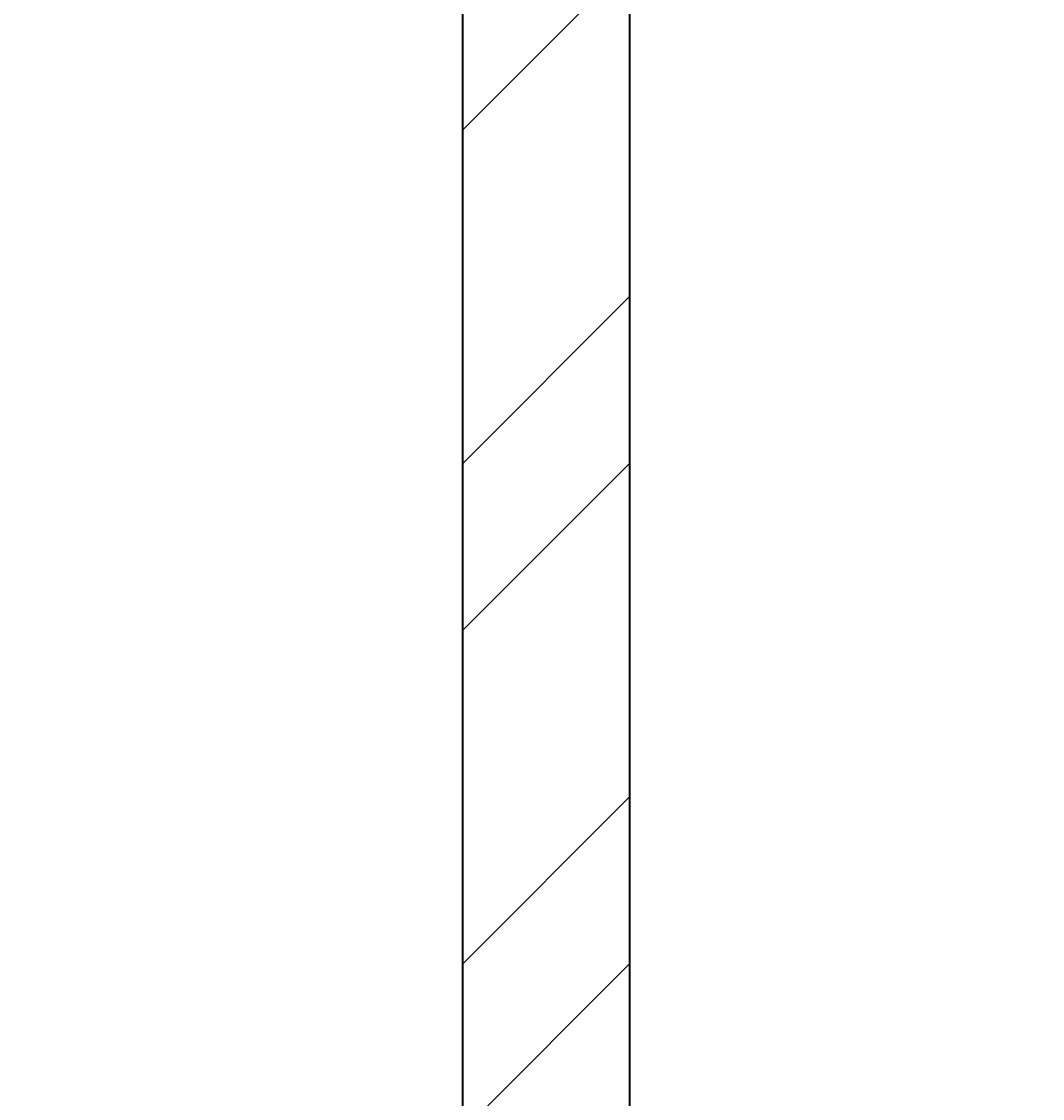
# Model space of a CAD drawing. Units: inches. Extents: x 1962 to 2771, y 1245 to 2660.
# Tile 63 of 114: x 2496 to 2523, y 2033 to 2062. Entities that reach past the tile are written whole.
import ezdxf

# ---------------------------------------------------------------- set-up
doc = ezdxf.new("R2010")
doc.units = ezdxf.units.IN
for name, color, linetype, lineweight in [('A-ANNO-DIMS', 2, 'Continuous', 18), ('A-WALL', 7, 'Continuous', 35), ('A-WALL-PATT', 252, 'Continuous', 13)]:
    doc.layers.add(name, color=color, linetype=linetype, lineweight=lineweight)
doc.styles.get("Standard").update_dxf_attribs({"font": 'arial.ttf'})
doc.dimstyles.get("Standard").update_dxf_attribs({"dimtxt": 0.18, "dimasz": 0.18, "dimexe": 0.18, "dimexo": 0.0625, "dimgap": 0.09, "dimtad": 0, "dimtih": 1, "dimtoh": 1, "dimdec": 4, "dimzin": 0, "dimdsep": 46, "dimtxsty": 'Standard', "dimcen": 0.09, "dimadec": 0, "dimazin": 0, "dimtfac": 1, "dimtdec": 4, "dimtofl": 0, "dimtmove": 0, "dimatfit": 3, "dimfxl": 1, "dimtolj": 1, "dimtzin": 0, "dimarcsym": 0})

# ---------------------------------------------------------------- blocks, each defined once
blk = doc.blocks.new('*D40')
at = {"layer": 'A-ANNO-DIMS', "color": 0, "lineweight": -2, "transparency": 16777216}
for p, q in [((2072.02, 2033.906), (2072.02, 2583.474)), ((2660.807, 2524.406), (2660.807, 2583.474)), ((2072.2, 2583.294), (2366.02, 2583.294)), ((2660.627, 2583.294), (2366.808, 2583.294))]:
    blk.add_line(p, q, dxfattribs=at)
at = {"layer": 'A-ANNO-DIMS', "color": 0, "transparency": 16777216}
for points in [[(2072.2, 2583.324), (2072.2, 2583.264), (2072.02, 2583.294)], [(2660.627, 2583.324), (2660.627, 2583.264), (2660.807, 2583.294)]]:
    blk.add_solid(points, dxfattribs=at)
at = {"layer": 'Defpoints', "color": 0, "transparency": 16777216}
for p in [(2660.807, 2583.294), (2660.807, 2524.344), (2072.02, 2033.844)]:
    blk.add_point(p, dxfattribs=at)
at = {"layer": 'A-ANNO-DIMS', "color": 0, "transparency": 16777216, "insert": (2366.414, 2583.294), "char_height": 0.18, "attachment_point": 5}
blk.add_mtext('\\A1;588.8', dxfattribs=at)

msp = doc.modelspace()

# ---------------------------------------------------------------- hatches: boundary and pattern name
at = {"layer": 'A-WALL-PATT'}
h = msp.add_hatch(dxfattribs=at)
h.set_pattern_fill('ANSI32', color=256)
h.paths.add_polyline_path([(2090.8074, 2467.3437), (2141.6481, 2467.3437), (2141.6481, 2469.5937), (2141.6481, 2471.8437), (2086.3074, 2471.8437), (2086.3074, 2422.5333), (2090.8074, 2422.5333)])
h.paths.add_polyline_path([(2282.7664, 2471.8437), (2204.8982, 2471.8437), (2204.8982, 2467.3437), (2234.8074, 2467.3437), (2234.8074, 2311.3437), (2228.7492, 2311.3437), (2228.7492, 2306.8437), (2234.8074, 2306.8437), (2331.9227, 2306.8437), (2331.9227, 2309.0937), (2331.9227, 2311.3437), (2239.3074, 2311.3437), (2239.3074, 2467.3437), (2282.7664, 2467.3437), (2282.7664, 2469.5937)])
h.paths.add_polyline_path([(2471.4531, 2519.8437), (2552.011, 2519.8437), (2564.3996, 2519.8437), (2564.3996, 2511.1389), (2568.8996, 2511.1389), (2568.8996, 2524.3437), (2466.9531, 2524.3437), (2466.9531, 2471.8437), (2450.0749, 2471.8437), (2446.4672, 2471.8437), (2446.4672, 2467.3437), (2450.0749, 2467.3437), (2475.9988, 2467.3437), (2475.9988, 2469.5937), (2475.9988, 2471.8437), (2471.4531, 2471.8437)])
h.paths.add_polyline_path([(2575.2231, 2469.5937), (2575.2231, 2471.8437), (2568.8996, 2471.8437), (2568.8996, 2487.1389), (2564.3996, 2487.1389), (2564.3996, 2471.8437), (2556.511, 2471.8437), (2499.2904, 2471.8437), (2499.2904, 2467.3437), (2507.8074, 2467.3437), (2507.8074, 2311.3437), (2414.863, 2311.3437), (2414.863, 2306.8437), (2512.3074, 2306.8437), (2517.0114, 2306.8437), (2517.0114, 2309.0937), (2517.0114, 2311.3437), (2512.3074, 2311.3437), (2512.3074, 2467.3437), (2575.2231, 2467.3437)])
h.paths.add_polyline_path([(2660.8074, 2471.8437), (2600.9602, 2471.8437), (2600.9602, 2467.3437), (2656.3074, 2467.3437), (2656.3074, 2432.5704), (2660.8074, 2432.5704)])
h.paths.add_polyline_path([(2660.8074, 2372.5704), (2656.3074, 2372.5704), (2656.3074, 2311.3437), (2600.276, 2311.3437), (2600.276, 2309.0937), (2600.276, 2306.8437), (2656.3074, 2306.8437), (2656.3074, 2296.2593), (2660.8074, 2296.2593)])
h.paths.add_polyline_path([(2572.3074, 2306.8437), (2577.1385, 2306.8437), (2577.1385, 2311.3437), (2551.082, 2311.3437), (2551.082, 2306.8437), (2567.8074, 2306.8437), (2567.8074, 2258.8437), (2540.0574, 2258.8437), (2540.0574, 2256.5937), (2540.0574, 2254.3437), (2567.8074, 2254.3437), (2656.3074, 2254.3437), (2656.3074, 2236.9085), (2660.8074, 2236.9085), (2660.8074, 2272.2593), (2656.3074, 2272.2593), (2656.3074, 2258.8437), (2572.3074, 2258.8437)])
h.paths.add_polyline_path([(2512.3074, 2254.3437), (2518.8716, 2254.3437), (2518.8716, 2256.5937), (2518.8716, 2258.8437), (2507.8074, 2258.8437), (2507.8074, 2177.8437), (2567.8074, 2177.8437), (2567.8074, 2172.9628), (2572.3074, 2172.9628), (2572.3074, 2177.8437), (2656.3074, 2177.8437), (2656.3074, 2166.4846), (2660.8074, 2166.4846), (2660.8074, 2200.9085), (2656.3074, 2200.9085), (2656.3074, 2182.3437), (2512.3074, 2182.3437)])
h.paths.add_polyline_path([(2656.3074, 2129.8437), (2572.3074, 2129.8437), (2572.3074, 2150.3044), (2570.0574, 2150.3044), (2567.8074, 2150.3044), (2567.8074, 2129.8437), (2507.8074, 2129.8437), (2507.8074, 2116.3027), (2510.0574, 2116.3027), (2512.3074, 2116.3027), (2512.3074, 2125.3437), (2567.8074, 2125.3437), (2572.3074, 2125.3437), (2656.3074, 2125.3437)])
h.paths.add_polyline_path([(2090.8074, 2362.5333), (2086.3074, 2362.5333), (2086.3074, 2298.6242), (2090.8074, 2298.6242), (2090.8074, 2306.8437), (2174.8074, 2306.8437), (2174.8074, 2286.4178), (2179.3074, 2286.4178), (2179.3074, 2306.8437), (2192.8641, 2306.8437), (2192.8641, 2309.0937), (2192.8641, 2311.3437), (2090.8074, 2311.3437)])
h.paths.add_polyline_path([(2209.156, 2258.8437), (2179.3074, 2258.8437), (2179.3074, 2263.2236), (2177.0574, 2263.2236), (2174.8074, 2263.2236), (2174.8074, 2258.8437), (2090.8074, 2258.8437), (2090.8074, 2274.6242), (2086.3074, 2274.6242), (2086.3074, 2238.2967), (2088.5574, 2238.2967), (2090.8074, 2238.2967), (2090.8074, 2254.3437), (2209.156, 2254.3437)])
h.paths.add_polyline_path([(2090.8074, 2177.8437), (2234.8074, 2177.8437), (2234.8074, 2173.1428), (2239.3074, 2173.1428), (2239.3074, 2258.8437), (2230.8442, 2258.8437), (2230.8442, 2256.5937), (2230.8442, 2254.3437), (2234.8074, 2254.3437), (2234.8074, 2182.3437), (2090.8074, 2182.3437), (2090.8074, 2202.2967), (2086.3074, 2202.2967), (2086.3074, 2140.0389), (2090.8074, 2140.0389)])
h.paths.add_polyline_path([(2090.8074, 2080.0389), (2086.3074, 2080.0389), (2086.3074, 2033.8437), (2090.8074, 2033.8437)], flags=17)
h.paths.add_polyline_path([(2244.9405, 2033.8437), (2239.3074, 2033.8437), (2239.3074, 2142.0665), (2237.2592, 2142.0665), (2234.8074, 2142.0665), (2234.8074, 2033.8437), (2090.8074, 2033.8437), (2076.5204, 2033.8437), (2072.0204, 2033.8437), (2072.0204, 2000.4493), (2076.5204, 2000.4493), (2076.5204, 2029.3437), (2090.8074, 2029.3437), (2244.9405, 2029.3437), (2244.9405, 2031.5937)])
h.paths.add_polyline_path([(2234.8074, 1933.3437), (2076.5204, 1933.3437), (2076.5204, 1952.4493), (2074.2704, 1952.4493), (2072.0204, 1952.4493), (2072.0204, 1933.3437), (2072.0204, 1928.8437), (2234.8074, 1928.8437)])
h.paths.add_polyline_path([(2090.8074, 1928.8437), (2086.3074, 1928.8437), (2086.3074, 1906.5013), (2090.8074, 1906.5013)])
h.paths.add_polyline_path([(2090.8074, 1846.5013), (2086.3074, 1846.5013), (2086.3074, 1769.9917), (2088.5574, 1769.9917), (2090.8074, 1769.9917), (2090.8074, 1780.3437), (2234.8074, 1780.3437), (2234.8074, 1708.3437), (2230.3764, 1708.3437), (2230.3764, 1703.8437), (2239.3074, 1703.8437), (2239.3074, 1792.6669), (2237.0574, 1792.6669), (2234.8074, 1792.6669), (2234.8074, 1784.8437), (2090.8074, 1784.8437)])
h.paths.add_polyline_path([(2239.3074, 1928.8437), (2244.9405, 1928.8437), (2244.9405, 1931.0937), (2244.9405, 1933.3437), (2234.8074, 1933.3437), (2234.8074, 1928.8437), (2234.8074, 1825.5949), (2239.3074, 1825.5949)])
h.paths.add_polyline_path([(2148.0425, 1649.0937), (2148.0425, 1651.3437), (2090.8074, 1651.3437), (2090.8074, 1646.8437), (2148.0425, 1646.8437)], flags=0)
h.paths.add_polyline_path([(2207.5601, 1708.3437), (2090.8074, 1708.3437), (2090.8074, 1703.8437), (2174.8074, 1703.8437), (2174.8074, 1651.3437), (2170.4457, 1651.3437), (2170.4457, 1646.8437), (2195.9924, 1646.8437), (2195.9924, 1649.0937), (2195.9924, 1651.3437), (2179.3074, 1651.3437), (2179.3074, 1703.8437), (2207.5601, 1703.8437), (2207.5601, 1706.0937)])
h.paths.add_polyline_path([(2090.8074, 1733.9917), (2086.3074, 1733.9917), (2086.3074, 1696.1032), (2088.5574, 1696.1032), (2090.8074, 1696.1032)])
h.paths.add_polyline_path([(2090.8074, 1672.1032), (2086.3074, 1672.1032), (2086.3074, 1600.3335), (2090.8074, 1600.3335)])
h.paths.add_polyline_path([(2090.8074, 1540.3335), (2086.3074, 1540.3335), (2086.3074, 1486.3437), (2139.6766, 1486.3437), (2139.6766, 1490.8437), (2090.8074, 1490.8437)])
h.paths.add_polyline_path([(2302.3876, 1490.8437), (2239.3074, 1490.8437), (2239.3074, 1646.8437), (2335.9994, 1646.8437), (2335.9994, 1651.3437), (2229.884, 1651.3437), (2229.884, 1646.8437), (2234.8074, 1646.8437), (2234.8074, 1490.8437), (2202.7103, 1490.8437), (2202.7103, 1488.5937), (2202.7103, 1486.3437), (2275.0699, 1486.3437), (2275.0699, 1475.772), (2279.5699, 1475.772), (2279.5699, 1486.3437), (2302.3876, 1486.3437)])
h.paths.add_polyline_path([(2279.5699, 1451.772), (2275.0699, 1451.772), (2275.0699, 1438.3437), (2174.8074, 1438.3437), (2174.8074, 1486.3437), (2179.7922, 1486.3437), (2179.7922, 1490.8437), (2163.3585, 1490.8437), (2163.3585, 1488.5937), (2163.3585, 1486.3437), (2170.3074, 1486.3437), (2170.3074, 1433.8437), (2279.5699, 1433.8437)])
h.paths.add_polyline_path([(2427.2363, 1490.8437), (2375.8074, 1490.8437), (2375.8074, 1646.8437), (2381.6401, 1646.8437), (2381.6401, 1651.3437), (2365.887, 1651.3437), (2365.887, 1649.0937), (2365.887, 1646.8437), (2371.3074, 1646.8437), (2371.3074, 1490.8437), (2327.5627, 1490.8437), (2327.5627, 1488.5937), (2327.5627, 1486.3437), (2371.3074, 1486.3437), (2371.3074, 1433.8437), (2375.8074, 1433.8437), (2375.8074, 1486.3437), (2427.2363, 1486.3437)])
h.paths.add_polyline_path([(2512.3074, 1646.8437), (2519.4351, 1646.8437), (2519.4351, 1649.0937), (2519.4351, 1651.3437), (2507.8074, 1651.3437), (2416.0063, 1651.3437), (2416.0063, 1649.0937), (2416.0063, 1646.8437), (2507.8074, 1646.8437), (2507.8074, 1490.8437), (2497.0532, 1490.8437), (2497.0532, 1488.5937), (2497.0532, 1486.3437), (2574.9344, 1486.3437), (2574.9344, 1476.0181), (2579.4344, 1476.0181), (2579.4344, 1486.3437), (2584.4872, 1486.3437), (2584.3074, 1490.8437), (2512.3074, 1490.8437)])
h.paths.add_polyline_path([(2470.5091, 1486.3437), (2473.9767, 1486.3437), (2473.9767, 1490.8437), (2449.6605, 1490.8437), (2449.6605, 1488.5937), (2449.6605, 1486.3437), (2466.0091, 1486.3437), (2466.0091, 1433.8437), (2470.5091, 1433.8437), (2579.4344, 1433.8437), (2579.4344, 1452.0181), (2574.9344, 1452.0181), (2574.9344, 1438.3437), (2554.5091, 1438.3437), (2470.5091, 1438.3437)])
h.paths.add_polyline_path([(2656.3074, 1490.8437), (2611.86, 1490.8437), (2611.86, 1486.3437), (2656.3074, 1486.3437)])
h.paths.add_polyline_path([(2660.8074, 1532.7007), (2658.5574, 1532.7007), (2656.3074, 1532.7007), (2656.3074, 1486.3437), (2660.8074, 1486.3437)])
h.paths.add_polyline_path([(2660.8074, 1664.9663), (2656.3074, 1664.9663), (2656.3074, 1651.3437), (2602.2313, 1651.3437), (2602.2313, 1646.8437), (2656.3074, 1646.8437), (2656.3074, 1592.7007), (2660.8074, 1592.7007)])
h.paths.add_polyline_path([(2660.8074, 1724.5221), (2656.3074, 1724.5221), (2656.3074, 1703.8437), (2542.4725, 1703.8437), (2542.4725, 1699.3437), (2567.8074, 1699.3437), (2567.8074, 1651.3437), (2552.7766, 1651.3437), (2552.7766, 1649.0937), (2552.7766, 1646.8437), (2577.2878, 1646.8437), (2577.2878, 1649.0937), (2577.2878, 1651.3437), (2572.3074, 1651.3437), (2572.3074, 1699.3437), (2656.3074, 1699.3437), (2656.3074, 1688.9663), (2660.8074, 1688.9663)])
h.paths.add_polyline_path([(2660.8074, 1880.6524), (2656.3074, 1880.6524), (2656.3074, 1832.8437), (2512.3074, 1832.8437), (2512.3074, 1837.8959), (2507.8074, 1837.8959), (2507.8074, 1828.3437), (2567.8074, 1828.3437), (2567.8074, 1804.3437), (2572.3074, 1804.3437), (2572.3074, 1828.3437), (2656.3074, 1828.3437), (2656.3074, 1818.6778), (2660.8074, 1818.6778)])
h.paths.add_polyline_path([(2660.8074, 1794.6778), (2656.3074, 1794.6778), (2656.3074, 1780.3437), (2572.3074, 1780.3437), (2572.3074, 1783.0303), (2570.0574, 1783.0303), (2567.8074, 1783.0303), (2567.8074, 1780.3437), (2507.8074, 1780.3437), (2507.8074, 1699.3437), (2517.8858, 1699.3437), (2517.8858, 1701.5937), (2517.8858, 1703.8437), (2512.3074, 1703.8437), (2512.3074, 1775.8437), (2656.3074, 1775.8437), (2656.3074, 1760.5221), (2660.8074, 1760.5221)])
h.paths.add_polyline_path([(2660.8074, 1981.3437), (2660.8074, 2020.2808), (2658.5574, 2020.2808), (2656.3074, 2020.2808), (2656.3074, 1981.3437), (2512.3074, 1981.3437), (2512.3074, 2086.6996), (2507.8074, 2086.6996), (2507.8074, 1981.3437), (2375.8074, 1981.3437), (2375.8074, 1986.8505), (2373.5574, 1986.8505), (2371.3074, 1986.8505), (2371.3074, 1973.2607), (2375.8074, 1973.2607), (2375.8074, 1976.8437), (2507.8074, 1976.8437), (2507.8074, 1865.4281), (2510.0574, 1865.4281), (2512.3074, 1865.4281), (2512.3074, 1976.8437), (2660.8074, 1976.8437)])
h.paths.add_polyline_path([(2375.8074, 1940.297), (2373.5574, 1940.297), (2371.3074, 1940.297), (2371.3074, 1933.3437), (2278.4434, 1933.3437), (2278.4434, 1928.8437), (2371.3074, 1928.8437), (2371.3074, 1651.3437), (2375.8074, 1651.3437)])
h.paths.add_polyline_path([(2660.8074, 1976.8437), (2656.3074, 1976.8437), (2656.3074, 1940.6524), (2660.8074, 1940.6524)], flags=17)
h.paths.add_polyline_path([(2660.8074, 2142.4846), (2656.3074, 2142.4846), (2656.3074, 2080.2808), (2660.8074, 2080.2808)])
h.paths.add_polyline_path([(2381.4189, 2311.3437), (2375.8074, 2311.3437), (2375.8074, 2467.3437), (2424.7242, 2467.3437), (2424.7242, 2469.5937), (2424.7242, 2471.8437), (2375.8074, 2471.8437), (2375.8074, 2524.3437), (2371.3074, 2524.3437), (2371.3074, 2471.8437), (2307.2097, 2471.8437), (2307.2097, 2467.3437), (2371.3074, 2467.3437), (2371.3074, 2311.3437), (2366.8901, 2311.3437), (2366.8901, 2306.8437), (2371.3074, 2306.8437), (2371.3074, 2033.8437), (2279.6589, 2033.8437), (2279.6589, 2029.3437), (2371.3074, 2029.3437), (2371.3074, 2014.2598), (2375.8074, 2014.2598), (2375.8074, 2306.8437), (2381.4189, 2306.8437)])
h.paths.add_polyline_path([(2263.3074, 2524.3437), (2170.3074, 2524.3437), (2170.3074, 2519.8437), (2170.3074, 2471.8437), (2165.0312, 2471.8437), (2165.0312, 2467.3437), (2179.6721, 2467.3437), (2179.6721, 2469.5161), (2179.6721, 2471.8437), (2174.8074, 2471.8437), (2174.8074, 2519.8437), (2258.8074, 2519.8437), (2258.8074, 2511.6436), (2263.3074, 2511.6436)])
h.paths.add_polyline_path([(2245.0232, 1361.4123), (2492.9468, 1361.4123), (2492.9468, 1398.505), (2245.0232, 1398.505)], flags=9)
h.paths.add_polyline_path([(2388.1434, 2086.6936), (2425.0704, 2086.6936), (2425.0704, 2105.3509), (2388.1434, 2105.3509)], flags=9)
h.paths.add_polyline_path([(2404.922, 2242.6744), (2445.7337, 2242.6744), (2445.7337, 2261.3318), (2404.922, 2261.3318)], flags=9)
h.paths.add_polyline_path([(2269.4107, 2156.7935), (2306.3378, 2156.7935), (2306.3378, 2175.4508), (2269.4107, 2175.4508)], flags=9)
h.paths.add_polyline_path([(2269.3277, 2233.4343), (2306.2547, 2233.4343), (2306.2547, 2252.0917), (2269.3277, 2252.0917)], flags=9)
h.paths.add_polyline_path([(2431.6052, 2320.6922), (2470.4456, 2320.6922), (2470.4456, 2339.3495), (2431.6052, 2339.3495)], flags=25)
h.paths.add_polyline_path([(2249.6902, 2315.7608), (2288.5306, 2315.7608), (2288.5306, 2334.4182), (2249.6902, 2334.4182)], flags=25)
h.paths.add_polyline_path([(2096.9301, 2314.3181), (2135.7704, 2314.3181), (2135.7704, 2332.9755), (2096.9301, 2332.9755)], flags=25)
h.paths.add_polyline_path([(2134.3475, 2285.7089), (2161.4655, 2285.7089), (2161.4655, 2304.3662), (2134.3475, 2304.3662)], flags=9)
h.paths.add_polyline_path([(2126.5155, 2209.4076), (2159.9227, 2209.4076), (2159.9227, 2228.065), (2126.5155, 2228.065)], flags=25)
h.paths.add_polyline_path([(2110.5753, 2141.5299), (2149.4157, 2141.5299), (2149.4157, 2160.1872), (2110.5753, 2160.1872)], flags=25)
h.paths.add_polyline_path([(2249.8618, 1968.3317), (2286.3966, 1968.3317), (2286.3966, 1986.989), (2249.8618, 1986.989)], flags=9)
h.paths.add_polyline_path([(2395.9507, 1777.0051), (2436.7624, 1777.0051), (2436.7624, 1795.6625), (2395.9507, 1795.6625)], flags=9)
h.paths.add_polyline_path([(2398.5259, 1888.5651), (2435.0062, 1888.5651), (2435.0062, 1907.2224), (2398.5259, 1907.2224)], flags=25)
h.paths.add_polyline_path([(2259.3506, 1728.3559), (2296.2776, 1728.3559), (2296.2776, 1747.0132), (2259.3506, 1747.0132)], flags=9)
h.paths.add_polyline_path([(2271.3698, 1845.268), (2308.2968, 1845.268), (2308.2968, 1863.9253), (2271.3698, 1863.9253)], flags=9)
h.paths.add_polyline_path([(2120.9355, 1786.3027), (2159.7759, 1786.3027), (2159.7759, 1804.9601), (2120.9355, 1804.9601)], flags=25)
h.paths.add_polyline_path([(2121.3164, 1732.1043), (2154.7236, 1732.1043), (2154.7236, 1750.7616), (2121.3164, 1750.7616)], flags=25)
h.paths.add_polyline_path([(2118.3706, 1678.8997), (2147.5282, 1678.8997), (2147.5282, 1697.557), (2118.3706, 1697.557)], flags=25)
h.paths.add_polyline_path([(2385.9227, 1493.557), (2424.763, 1493.557), (2424.763, 1512.2143), (2385.9227, 1512.2143)], flags=25)
h.paths.add_polyline_path([(2248.7058, 1500.0256), (2287.5462, 1500.0256), (2287.5462, 1518.6829), (2248.7058, 1518.6829)], flags=25)
h.paths.add_polyline_path([(2104.1669, 1617.3771), (2143.0073, 1617.3771), (2143.0073, 1636.0344), (2104.1669, 1636.0344)], flags=9)
h.paths.add_polyline_path([(2096.0714, 1447.8824), (2137.3845, 1447.8824), (2137.3845, 1458.1859), (2096.0714, 1458.1859)], flags=9)
h.paths.add_polyline_path([(2180.6114, 1440.325), (2209.7689, 1440.325), (2209.7689, 1458.9823), (2180.6114, 1458.9823)], flags=25)
h.paths.add_polyline_path([(2316.1698, 1447.9637), (2357.4829, 1447.9637), (2357.4829, 1458.2673), (2316.1698, 1458.2673)], flags=9)
h.paths.add_polyline_path([(2397.6187, 1447.9637), (2438.9318, 1447.9637), (2438.9318, 1458.2673), (2397.6187, 1458.2673)], flags=9)
h.paths.add_polyline_path([(2473.0778, 1439.5953), (2502.2354, 1439.5953), (2502.2354, 1458.2527), (2473.0778, 1458.2527)], flags=25)
h.paths.add_polyline_path([(2589.7027, 1447.8819), (2631.0158, 1447.8819), (2631.0158, 1458.1855), (2589.7027, 1458.1855)], flags=9)
h.paths.add_polyline_path([(2522.4009, 1497.5285), (2561.2413, 1497.5285), (2561.2413, 1516.1859), (2522.4009, 1516.1859)], flags=25)
h.paths.add_polyline_path([(2579.6565, 1671.3482), (2608.8141, 1671.3482), (2608.8141, 1690.0056), (2579.6565, 1690.0056)], flags=25)
h.paths.add_polyline_path([(2544.7038, 1725.5064), (2578.1111, 1725.5064), (2578.1111, 1744.1637), (2544.7038, 1744.1637)], flags=25)
h.paths.add_polyline_path([(2578.1191, 1807.472), (2607.2766, 1807.472), (2607.2766, 1826.1293), (2578.1191, 1826.1293)], flags=25)
h.paths.add_polyline_path([(2595.0614, 1835.1839), (2633.9018, 1835.1839), (2633.9018, 1853.8413), (2595.0614, 1853.8413)], flags=25)
h.paths.add_polyline_path([(2567.0097, 2097.7035), (2605.8501, 2097.7035), (2605.8501, 2116.3609), (2567.0097, 2116.3609)], flags=9)
h.paths.add_polyline_path([(2586.644, 2134.6454), (2615.8015, 2134.6454), (2615.8015, 2153.3027), (2586.644, 2153.3027)], flags=9)
h.paths.add_polyline_path([(2544.6185, 2212.6783), (2578.0258, 2212.6783), (2578.0258, 2231.3356), (2544.6185, 2231.3356)], flags=25)
h.paths.add_polyline_path([(2577.0273, 2256.9023), (2606.1849, 2256.9023), (2606.1849, 2275.5597), (2577.0273, 2275.5597)], flags=24)
h.paths.add_polyline_path([(2605.2683, 2315.2821), (2644.1087, 2315.2821), (2644.1087, 2333.9395), (2605.2683, 2333.9395)], flags=25)
h.paths.add_polyline_path([(2583.1244, 2496.1815), (2624.4375, 2496.1815), (2624.4375, 2506.4851), (2583.1244, 2506.4851)], flags=9)
h.paths.add_polyline_path([(2474.761, 2497.0823), (2503.9185, 2497.0823), (2503.9185, 2515.7397), (2474.761, 2515.7397)], flags=25)
h.paths.add_polyline_path([(2387.5787, 2494.2563), (2428.902, 2494.2563), (2428.902, 2504.5598), (2387.5787, 2504.5598)], flags=9)
h.paths.add_polyline_path([(2300.1657, 2500.1564), (2341.4788, 2500.1564), (2341.4788, 2510.46), (2300.1657, 2510.46)], flags=25)
h.paths.add_polyline_path([(2176.8589, 2497.5843), (2206.0165, 2497.5843), (2206.0165, 2516.2416), (2176.8589, 2516.2416)], flags=25)
h.paths.add_polyline_path([(2097.4668, 2494.9762), (2138.7799, 2494.9762), (2138.7799, 2505.2798), (2097.4668, 2505.2798)], flags=9)

# ---------------------------------------------------------------- linework, layer by layer
at = {"layer": 'A-WALL'}
for p, q in [((2512.3074, 2088.0256), (2512.3074, 1981.3437)), ((2507.8074, 2086.6996), (2507.8074, 1981.3437)), ((2507.8074, 2086.6996), (2507.8074, 1981.3437))]:
    msp.add_line(p, q, dxfattribs=at)

# ---------------------------------------------------------------- dimensions: what is measured, and where the dimension line sits
at = {"layer": 'A-ANNO-DIMS'}
dim = msp.add_linear_dim(base=(2660.8074, 2583.2937), p1=(2072.0204, 2033.8437), p2=(2660.8074, 2524.3437), dimstyle='Standard', override={"dimdec": 1, "dimlfac": 1, "dimrnd": 0, "dimzin": 0, "dimdsep": 46, "dimlunit": 2}, dxfattribs=at)
dim.commit()
dim.dimension.update_dxf_attribs({"geometry": '*D40', "text_midpoint": (2366.4139, 2583.2937)})

doc.saveas('drawing.dxf')
